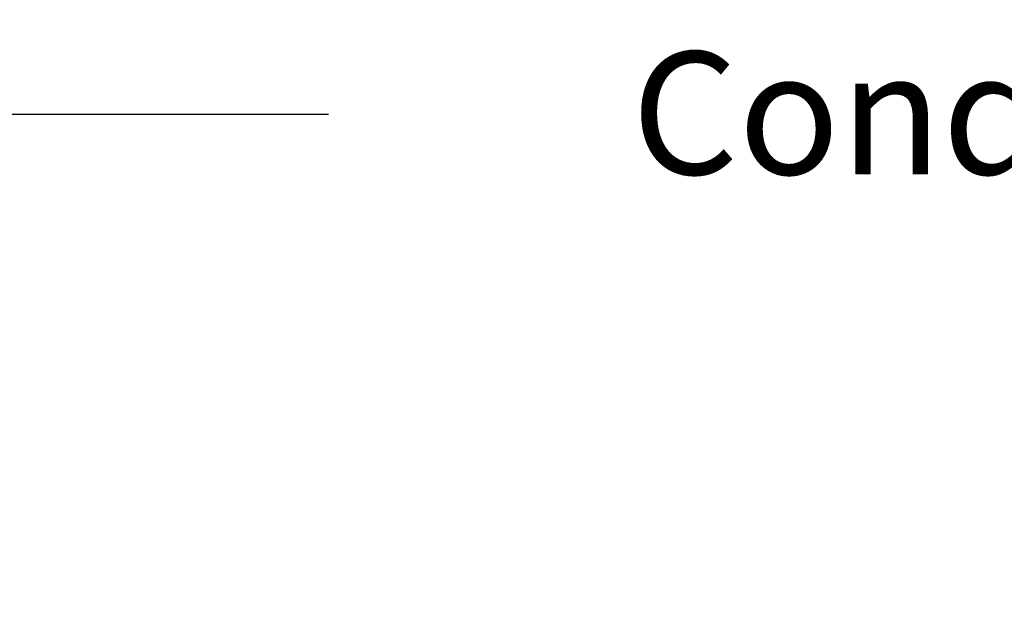
# Model space of a CAD drawing. Units: inches. Extents: x -12 to 334, y -10 to 186.
# Tile 10 of 77: x 74 to 106, y -6 to 13. Entities that reach past the tile are written whole.
import ezdxf
from ezdxf import colors
from ezdxf.entities.mleader import LeaderData, LeaderLine
from ezdxf.math import Vec2, Vec3

# ---------------------------------------------------------------- set-up
doc = ezdxf.new("R2010")
doc.units = ezdxf.units.IN
doc.header["$MEASUREMENT"] = 0
doc.layers.add('M-ANNO-TEXT', color=3, linetype='Continuous', lineweight=25)
doc.styles.get("Standard").update_dxf_attribs({"font": 'arial.ttf'})

msp = doc.modelspace()

# ---------------------------------------------------------------- leaders
at = {"layer": 'M-ANNO-TEXT'}
ml = msp.add_multileader_mtext('Standard', dxfattribs=at)
ml.set_content('^ICondensate outlet', color=256)
ml.set_leader_properties()
ml.build(insert=Vec2(0, 0))
ml.multileader.update_dxf_attribs({"dogleg_length": 0.36, "arrow_head_size": 0.7})
ctx = ml.context
ctx.base_point, ctx.arrow_head_size, ctx.landing_gap_size, ctx.plane_origin = Vec3(83.8784, 10.3512), 0.7, 0.09, Vec3(49.4251, 25.7584)
notes = []
notes.append((ctx, [(0, (1, 1, 0), (70.8242, 10.3512), (1, 0), 13.0542, [(0, [(42.9275, 33.6752)], 0, [])])]))
ctx.mtext.insert, ctx.mtext.flow_direction = Vec3(83.9684, 12.3853), 5
for ctx, leaders in notes:
    for number, flags, end, landing, length, lines in leaders:
        leader = LeaderData()
        leader.index, (leader.has_last_leader_line, leader.has_dogleg_vector, leader.attachment_direction) = number, flags
        leader.last_leader_point, leader.dogleg_vector, leader.dogleg_length = Vec3(end), Vec3(landing), length
        for number, points, colour, breaks in lines:
            line = LeaderLine()
            line.index, line.vertices, line.color, line.breaks = number, Vec3.list(points), colors.encode_raw_color(colour), breaks
            leader.lines.append(line)
        ctx.leaders.append(leader)

doc.saveas('drawing.dxf')
